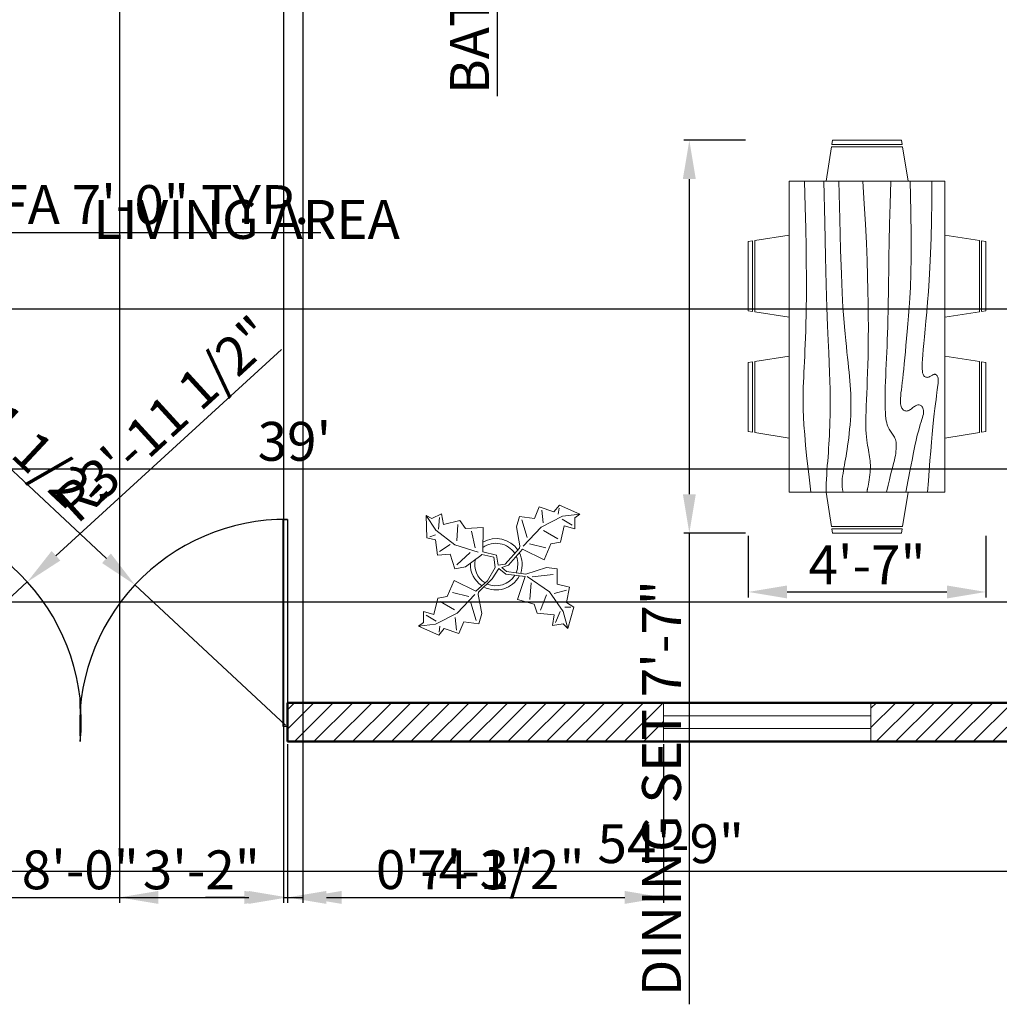
# Model space of a CAD drawing. Units: inches. Extents: x 61993 to 62774, y 55335 to 55871.
# Tile 2 of 6: x 62247 to 62474, y 55335 to 55563. Entities that reach past the tile are written whole.
import ezdxf

# ---------------------------------------------------------------- set-up
doc = ezdxf.new("R2010")
doc.units = ezdxf.units.IN
for name, color, linetype, lineweight in [('A-ANNO-DIMS', 2, 'Continuous', 18), ('A-AREA-IDEN', 7, 'Continuous', 25), ('A-DOOR', 3, 'Continuous', 25), ('A-FURN', 9, 'Continuous', 18), ('A-FURN-PLNT', 94, 'Continuous', 13), ('A-GLAZ', 4, 'Continuous', 18), ('A-WALL', 7, 'Continuous', 50)]:
    doc.layers.add(name, color=color, linetype=linetype, lineweight=lineweight)
doc.layers.add('A-WALL-PATT', color=40, linetype='Continuous', lineweight=13, true_color=0xf8d731)
doc.styles.get("Standard").update_dxf_attribs({"font": 'arial.ttf'})
doc.dimstyles.new('ISO-25', dxfattribs={"dimtxt": 9, "dimasz": 9, "dimexe": 1.25, "dimexo": 0.625, "dimtad": 1, "dimdec": 1, "dimrnd": 9, "dimlunit": 3, "dimtxsty": 'Standard', "dimcen": 2.5, "dimadec": 0, "dimazin": 0, "dimtfac": 1, "dimtdec": 1, "dimtmove": 0, "dimatfit": 3, "dimfxl": 1, "dimarcsym": 0})

# ---------------------------------------------------------------- blocks, each defined once
blk = doc.blocks.new('*D12')
at = {"layer": 'A-ANNO-DIMS', "color": 0, "lineweight": -2, "transparency": 16777216}
for p, q in [((62077.82, 55405.58), (62077.82, 55460.37)), ((62086.82, 55459.12), (62534.69, 55459.12)), ((62543.69, 55405.58), (62543.69, 55460.37))]:
    blk.add_line(p, q, dxfattribs=at)
at = {"layer": 'A-ANNO-DIMS', "color": 0, "transparency": 16777216}
for points in [[(62086.82, 55460.62), (62086.82, 55457.62), (62077.82, 55459.12)], [(62534.69, 55460.62), (62534.69, 55457.62), (62543.69, 55459.12)]]:
    blk.add_solid(points, dxfattribs=at)
at = {"layer": 'Defpoints', "color": 0, "transparency": 16777216}
for p in [(62543.69, 55459.12), (62077.82, 55404.96), (62543.69, 55404.96)]:
    blk.add_point(p, dxfattribs=at)
at = {"layer": 'A-ANNO-DIMS', "color": 0, "transparency": 16777216, "insert": (62310.76, 55464.35), "char_height": 9, "attachment_point": 5}
blk.add_mtext("39'", dxfattribs=at)
blk = doc.blocks.new('Plant - Rubber or Philodendron')
for p, q in [((13.3837, 12.301), (14.68, 13.9039)), ((14.68, 13.9039), (19.3848, 11.8146)), ((-16.2005, 11.4774), (-13.9899, 8.1064)), ((-16.2005, 11.4774), (-14.8639, 10.7964)), ((-16.0159, 6.3329), (-16.2005, 11.4774)), ((-14.8639, 10.7964), (-12.6195, 11.8975)), ((-12.6195, 11.8975), (-12.1909, 9.4345)), ((8.8871, 10.7908), (9.9809, 13.4933)), ((9.9809, 13.4933), (13.3837, 12.301)), ((10.5828, 12.6946), (10.8893, 9.7953)), ((14.5816, 13.2037), (14.3848, 11.8033)), ((19.3848, 11.8146), (15.3859, 11.3055)), ((19.3848, 11.8146), (18.1868, 10.9119)), ((-13.3174, 8.325), (-13.0735, 11.0065)), ((-12.1909, 9.4345), (-8.3829, 10.3)), ((-8.8369, 9.409), (-9.0894, 5.6095)), ((-8.3829, 10.3), (-7.0549, 8.501)), ((4.6914, 8.8812), (5.3859, 11.2828)), ((5.3859, 11.2828), (8.8871, 10.7908)), ((5.9878, 10.4842), (7.1971, 6.3869)), ((15.3859, 11.3055), (10.3916, 8.7942)), ((15.2875, 10.6053), (17.5907, 9.2105)), ((18.1868, 10.9119), (18.1925, 8.4119)), ((-15.3434, 6.5514), (-13.9984, 6.9884)), ((-13.9899, 8.1064), (-9.5434, 4.7185)), ((-7.0549, 8.501), (-3.0284, 8.6941)), ((-4.8529, 4.012), (-5.7184, 7.82)), ((-3.0284, 8.6941), (-3.0709, 3.1041)), ((4.6914, 8.8812), (5.5014, 4.4831)), ((10.3916, 8.7942), (6.2847, 4.4028)), ((14.2977, 6.1031), (10.9934, 7.9956)), ((15.7909, 9.1065), (14.8995, 5.3044)), ((18.1925, 8.4119), (15.7909, 9.1065)), ((-14.0069, 5.8704), (-16.0159, 6.3329)), ((-13.5868, 2.2894), (-14.0069, 5.8704)), ((-13.1329, 3.1804), (-10.6614, 4.727)), ((-9.5434, 4.7185), (-4.1917, 2.9888)), ((7.7005, 4.8881), (11.5025, 3.9967)), ((12.7005, 4.8994), (11.1089, 1.1958)), ((14.8995, 5.3044), (12.7005, 4.8994)), ((-10.6784, 2.491), (-13.5868, 2.2894)), ((-9.5858, -0.8715), (-10.6784, 2.491)), ((-9.1318, 0.0195), (-5.9793, 2.9025)), ((-3.5248, 2.2131), (-3.3011, 2.4355)), ((-3.3011, 2.4355), (-0.5306, 1.7947)), ((-3.0709, 3.1041), (0.0797, 2.3163)), ((0.0797, 2.3163), (0.4866, -0.031)), ((2.1141, 0.2298), (5.4346, 3.9146)), ((6.1032, 3.6844), (2.8262, -0.031)), ((5.4346, 3.9146), (5.5014, 4.4831)), ((11.1089, 1.1958), (6.1032, 3.6844)), ((-7.1228, -0.443), (-3.5248, 2.2131)), ((-0.5306, 1.7947), (-0.2255, -0.5527)), ((-0.5306, 1.7947), (-0.5306, 1.7947)), ((0.4866, -0.031), (2.1141, 0.2298)), ((-7.1228, -0.443), (-9.5858, -0.8715)), ((-2.019, -3.6148), (-0.2255, -0.5527)), ((-0.9375, -3.1608), (0.5883, -0.8135)), ((0.5883, -0.8135), (2.2447, -2.0916)), ((2.8262, -0.031), (1.3003, -0.5527)), ((1.3003, -0.5527), (2.4193, -1.4655)), ((2.2447, -2.0916), (6.7108, -2.6626)), ((2.4193, -1.4655), (6.895, -2.1175)), ((11.6605, -0.5413), (6.895, -2.1175)), ((8.3544, -2.7453), (13.1973, -2.1704)), ((11.6605, -0.5413), (14.1354, -0.8948)), ((14.1354, -0.8948), (14.1354, -4.4304)), ((-11.3237, -7.2629), (-9.7321, -3.5593)), ((-9.7321, -3.5593), (-4.7264, -6.0479)), ((-2.019, -3.6148), (-4.7264, -6.0479)), ((-4.0579, -6.2781), (-0.9375, -3.1608)), ((4.943, -7.9659), (6.7108, -2.6626)), ((12.3677, -6.1981), (7.219, -2.6772)), ((8.125, -4.0768), (7.7715, -7.9659)), ((14.1354, -4.4304), (16.9638, -5.1375)), ((-6.3237, -7.2516), (-10.1257, -6.3602)), ((-9.0148, -11.1577), (-4.9047, -6.8122)), ((-4.1246, -6.8466), (-4.0579, -6.2781)), ((15.5496, -10.7943), (12.3677, -6.1981)), ((16.2567, -5.8446), (13.4283, -6.5517)), ((16.9638, -5.1375), (16.2567, -8.673)), ((-14.4141, -11.4699), (-13.5228, -7.6679)), ((-13.5228, -7.6679), (-11.3237, -7.2629)), ((-12.921, -8.4665), (-9.6166, -10.359)), ((-4.611, -12.8477), (-5.8203, -8.7504)), ((-3.3146, -11.2447), (-4.1246, -6.8466)), ((8.8321, -9.0266), (4.943, -7.9659)), ((9.5392, -11.1479), (8.8321, -9.0266)), ((10.2463, -10.4408), (11.6605, -6.9053)), ((16.2567, -8.673), (18.0245, -9.7337)), ((-16.8157, -10.7754), (-14.4141, -11.4699)), ((-16.8101, -13.2754), (-16.8157, -10.7754)), ((-14.0091, -13.669), (-9.0148, -11.1577)), ((-3.3146, -11.2447), (-4.0092, -13.6463)), ((13.4283, -11.5015), (9.5392, -11.1479)), ((14.8425, -10.7943), (13.7819, -13.2692)), ((16.6103, -14.6834), (15.5496, -10.7943)), ((17.3174, -9.7337), (15.9032, -9.7337)), ((18.0245, -9.7337), (16.6103, -14.6834)), ((-18.008, -14.1781), (-16.8101, -13.2754)), ((-18.008, -14.1781), (-14.0091, -13.669)), ((-13.9107, -12.9688), (-16.2139, -11.574)), ((-9.206, -15.0581), (-9.5126, -12.1588)), ((-7.5103, -13.1543), (-8.6042, -15.8568)), ((-4.0092, -13.6463), (-7.5103, -13.1543)), ((13.0748, -13.9763), (13.4283, -11.5015)), ((15.5496, -13.6228), (13.0748, -13.9763)), ((16.6103, -14.6834), (15.5496, -13.6228)), ((-13.3032, -16.2674), (-18.008, -14.1781)), ((-12.0069, -14.6645), (-13.3032, -16.2674)), ((-13.2048, -15.5672), (-13.008, -14.1668)), ((-8.6042, -15.8568), (-12.0069, -14.6645))]:
    blk.add_line(p, q)
for centre, radius, start, end in [((0, 0), 6.1275, 34.37569, 120.1028), ((-0.0601, -0.2075), 5.2461, 33.82192, 124.9414), ((-0.098, 0.1364), 6.1288, 341.2017, 26.09184), ((0.0308, 0.1664), 6, 178.6147, 235.1169), ((0.0308, 0.1664), 5, 168.1647, 238.6725), ((-0.2664, 0.1682), 5.2775, 338.4094, 20.03007), ((-0.0234, 0.3825), 6.1492, 242.5812, 331.2714), ((-0.1102, 0.4886), 5.2883, 247.3711, 327.472)]:
    blk.add_arc(centre, radius, start, end)
blk = doc.blocks.new('Dining Set - 36 x 72 in.')
for p, q in [((-22, 27.5), (-22.1562, 26.50042)), ((-22, 27.5), (-6, 27.5)), ((-5.8437, 26.49966), (-6, 27.5)), ((6, 27.5), (5.8438, 26.50042)), ((6, 27.5), (22, 27.5)), ((22.1563, 26.49966), (22, 27.5)), ((-22.2343, 26.00059), (-23.4847, 17.99762)), ((-22.2304, 26), (-5.7608, 26)), ((-5.8416, 26.5), (-22.1534, 26.5)), ((-4.5152, 17.99762), (-5.7655, 25.99926)), ((5.7657, 26.00059), (4.5153, 17.99762)), ((5.7696, 26), (22.2392, 26)), ((22.1584, 26.5), (5.8466, 26.5)), ((23.4848, 17.99762), (22.2345, 25.99926)), ((36, 18), (-36, 18)), ((-36, 18), (-36, -18)), ((36, -18), (36, 18)), ((-44.0006, 8.23428), (-35.9976, 9.48474)), ((44.0006, 8.23428), (35.9976, 9.48474)), ((-45.5, 8), (-44.5004, 8.15617)), ((-45.5, 8), (-45.5, -8)), ((-44.5, -8.15843), (-44.5, 8.15338)), ((-44, 8.23041), (-44, -8.23915)), ((44, 8.23041), (44, -8.23915)), ((44.5, -8.15843), (44.5, 8.15338)), ((45.5, 8), (44.5005, 8.15617)), ((45.5, 8), (45.5, -8)), ((-44.4997, -8.15631), (-45.5, -8)), ((-35.9976, -9.48476), (-43.9993, -8.2345)), ((35.9976, -9.48476), (43.9993, -8.2345)), ((44.4997, -8.15631), (45.5, -8)), ((-36, -18), (36, -18)), ((-22.2343, -26.0006), (-23.4847, -17.99762)), ((-4.5152, -17.99762), (-5.7655, -25.99928)), ((5.7657, -26.0006), (4.5153, -17.99762)), ((23.4848, -17.99762), (22.2345, -25.99928)), ((-22.2304, -26), (-5.7608, -26)), ((-22, -27.5), (-22.1562, -26.50044)), ((-5.8416, -26.5), (-22.1534, -26.5)), ((-5.8437, -26.49967), (-6, -27.5)), ((5.7696, -26), (22.2392, -26)), ((6, -27.5), (5.8438, -26.50044)), ((22.1584, -26.5), (5.8466, -26.5)), ((22.1563, -26.49967), (22, -27.5)), ((-22, -27.5), (-6, -27.5)), ((6, -27.5), (22, -27.5))]:
    blk.add_line(p, q)
for points in [[(-36, 15), (-31.1772, 14.97754), (-26.8079, 14.91406), (-22.8538, 14.81543), (-19.276, 14.6875), (-16.0362, 14.53613), (-13.0957, 14.36718), (-10.4159, 14.18652), (-7.9583, 14), (-5.6904, 13.81315), (-3.6035, 13.63021), (-1.6954, 13.45508), (0.0365, 13.29166), (1.5945, 13.14388), (2.9811, 13.01562), (4.1988, 12.9108), (5.25, 12.83333), (6.1393, 12.78613), (6.8802, 12.76823), (7.4883, 12.77767), (7.9792, 12.8125), (8.3685, 12.87077), (8.6719, 12.95052), (8.9049, 13.0498), (9.0833, 13.16666), (9.2205, 13.29899), (9.3216, 13.44401), (9.3895, 13.59879), (9.4271, 13.76041), (9.4373, 13.92594), (9.4232, 14.09245), (9.3875, 14.257), (9.3333, 14.41666), (9.2638, 14.56917), (9.1836, 14.71484), (9.0975, 14.85465), (9.0104, 14.98958), (8.9272, 15.1206), (8.8529, 15.2487), (8.7922, 15.37483), (8.75, 15.5), (8.7305, 15.62467), (8.7344, 15.74739), (8.7617, 15.86621), (8.8125, 15.97916), (8.8867, 16.08431), (8.9844, 16.17968), (9.1055, 16.26334), (9.25, 16.33333), (9.4189, 16.38802), (9.6172, 16.42708), (9.8506, 16.45052), (10.125, 16.45833), (10.4463, 16.45052), (10.8203, 16.42708), (11.2529, 16.38802), (11.75, 16.33333), (12.3184, 16.26318), (12.9694, 16.17838), (13.7151, 16.07991), (14.5677, 15.96875), (15.5395, 15.84586), (16.6426, 15.71224), (17.8893, 15.56884), (19.2917, 15.41666), (20.859, 15.25667), (22.5879, 15.08984), (24.4721, 14.91715), (26.5052, 14.73958), (28.6809, 14.5581), (30.9929, 14.3737), (33.4347, 14.18733), (36, 14)], [(-36, 10), (-28.9766, 10.14274), (-23.1725, 10.20442), (-18.4241, 10.19775), (-14.5677, 10.13541), (-11.4399, 10.03011), (-8.877, 9.89453), (-6.7154, 9.74137), (-4.7917, 9.58333), (-2.9698, 9.43082), (-1.2246, 9.28515), (0.4415, 9.14534), (2.026, 9.01041), (3.5266, 8.87939), (4.9408, 8.7513), (6.266, 8.62516), (7.5, 8.5), (8.6411, 8.37549), (9.6914, 8.2539), (10.6538, 8.13818), (11.5312, 8.03125), (12.3267, 7.93603), (13.043, 7.85547), (13.6831, 7.79248), (14.25, 7.75), (14.7471, 7.7303), (15.1797, 7.73307), (15.5537, 7.75732), (15.875, 7.80208), (16.1494, 7.86637), (16.3828, 7.94922), (16.5811, 8.04964), (16.75, 8.16666), (16.8944, 8.29915), (17.0143, 8.44531), (17.1089, 8.60319), (17.1771, 8.77083), (17.218, 8.94629), (17.2305, 9.1276), (17.2137, 9.31282), (17.1667, 9.5), (17.0895, 9.6875), (16.987, 9.875), (16.8649, 10.0625), (16.7292, 10.25), (16.5856, 10.4375), (16.4401, 10.625), (16.2985, 10.8125), (16.1667, 11), (16.05, 11.18733), (15.9518, 11.3737), (15.8752, 11.5581), (15.8229, 11.73958), (15.798, 11.91715), (15.8034, 12.08984), (15.842, 12.25667), (15.9167, 12.41666), (16.0295, 12.56836), (16.1784, 12.70833), (16.3605, 12.83268), (16.5729, 12.9375), (16.8127, 13.01888), (17.0768, 13.07291), (17.3625, 13.0957), (17.6667, 13.08333), (17.9894, 13.03312), (18.3418, 12.94726), (18.7382, 12.82918), (19.1927, 12.68229), (19.7195, 12.51001), (20.3327, 12.31575), (21.0465, 12.10294), (21.875, 11.875), (22.8357, 11.63354), (23.959, 11.37304), (25.2786, 11.08618), (26.8282, 10.76562), (28.6414, 10.40405), (30.752, 9.99414), (33.1936, 9.52856), (36, 9)], [(-36, 5.5), (-30.7157, 5.3348), (-26.069, 5.20963), (-21.9946, 5.11767), (-18.4271, 5.05208), (-15.3009, 5.00602), (-12.5508, 4.97265), (-10.1112, 4.94515), (-7.9167, 4.91666), (-5.909, 4.88167), (-4.0586, 4.83984), (-2.3429, 4.79215), (-0.7396, 4.73958), (0.7739, 4.6831), (2.22, 4.6237), (3.6213, 4.56233), (5, 4.5), (6.373, 4.43782), (7.7344, 4.3776), (9.0723, 4.32129), (10.375, 4.27083), (11.6309, 4.22819), (12.8281, 4.19531), (13.9551, 4.17415), (15, 4.16666), (15.954, 4.17448), (16.819, 4.19791), (17.6001, 4.23698), (18.3021, 4.29166), (18.9299, 4.36198), (19.4883, 4.44791), (19.9823, 4.54948), (20.4167, 4.66666), (20.7969, 4.79899), (21.1302, 4.94401), (21.4245, 5.09879), (21.6875, 5.26041), (21.9271, 5.42594), (22.1511, 5.59245), (22.3672, 5.757), (22.5834, 5.91666), (22.8065, 6.06868), (23.0404, 6.21093), (23.2879, 6.34147), (23.5521, 6.45833), (23.8358, 6.55957), (24.142, 6.64323), (24.4735, 6.70735), (24.8334, 6.75), (25.2235, 6.76969), (25.642, 6.76692), (26.0858, 6.74267), (26.5521, 6.69791), (27.0379, 6.63362), (27.5404, 6.55078), (28.0565, 6.45036), (28.5834, 6.33333), (29.1242, 6.19987), (29.7071, 6.04687), (30.3661, 5.87044), (31.1354, 5.66666), (32.0493, 5.43164), (33.142, 5.16146), (34.4475, 4.85221), (36, 4.5)], [(-36, -1), (-30.7915, -0.6591), (-26.0195, -0.38216), (-21.6519, -0.16284), (-17.6563, 0.00521), (-14.0005, 0.12833), (-10.6523, 0.21289), (-7.5796, 0.26522), (-4.75, 0.29166), (-2.134, 0.29793), (0.2878, 0.28711), (2.5317, 0.26163), (4.6146, 0.22396), (6.5529, 0.17651), (8.3633, 0.12174), (10.0623, 0.06209), (11.6667, 0), (13.1899, -0.06201), (14.6341, -0.1211), (15.9982, -0.17432), (17.2813, -0.21875), (18.4823, -0.25147), (19.6003, -0.26953), (20.6343, -0.27002), (21.5834, -0.25), (22.4481, -0.20768), (23.2357, -0.14584), (23.9549, -0.06836), (24.6146, 0.02083), (25.2235, 0.11784), (25.7904, 0.21875), (26.3241, 0.31966), (26.8334, 0.41666), (27.3265, 0.50618), (27.8099, 0.58593), (28.2894, 0.65397), (28.7709, 0.70833), (29.2601, 0.74707), (29.763, 0.76823), (30.2855, 0.76985), (30.8334, 0.75), (31.4088, 0.70784), (31.9994, 0.64713), (32.589, 0.57275), (33.1615, 0.48958), (33.7008, 0.4025), (34.1908, 0.3164), (34.6153, 0.23616), (34.9584, 0.16666), (35.2099, 0.11165), (35.3848, 0.07031), (35.504, 0.04069), (35.5886, 0.02083), (35.6594, 0.00879), (35.7377, 0.0026), (35.8442, 0.00032), (36, 0)], [(-36, -6.5), (-27.1843, -6.31267), (-20.084, -6.1263), (-14.469, -5.9419), (-10.1094, -5.76042), (-6.7752, -5.58285), (-4.2363, -5.41016), (-2.2629, -5.24333), (-0.625, -5.08334), (0.8708, -4.93099), (2.2715, -4.78646), (3.5872, -4.64974), (4.8281, -4.52084), (6.0046, -4.39974), (7.127, -4.28646), (8.2053, -4.18099), (9.25, -4.08334), (10.2705, -3.99382), (11.2734, -3.91407), (12.2647, -3.84603), (13.25, -3.79167), (14.2354, -3.75293), (15.2266, -3.73177), (16.2295, -3.73015), (17.25, -3.75), (18.2912, -3.79248), (19.3451, -3.85547), (20.4009, -3.93604), (21.4479, -4.03125), (22.4754, -4.13819), (23.4727, -4.25391), (24.4289, -4.37549), (25.3334, -4.5), (26.1785, -4.62492), (26.9694, -4.74935), (27.7145, -4.87281), (28.4219, -4.99479), (29.1, -5.11483), (29.7572, -5.23242), (30.4016, -5.34709), (31.0417, -5.45834), (31.6837, -5.56437), (32.3262, -5.65821), (32.9658, -5.73153), (33.599, -5.77604), (34.2224, -5.78345), (34.8327, -5.74545), (35.4264, -5.65373), (36, -5.5)], [(-36, -10), (-26.4022, -9.81299), (-18.4675, -9.62891), (-11.9839, -9.45069), (-6.7396, -9.28125), (-2.5226, -9.12354), (0.8789, -8.98047), (3.6769, -8.85498), (6.0833, -8.75), (8.2767, -8.66765), (10.3021, -8.60677), (12.1712, -8.56543), (13.8958, -8.54167), (15.4876, -8.53353), (16.9583, -8.53907), (18.3197, -8.55632), (19.5834, -8.58334), (20.7616, -8.61841), (21.8685, -8.66081), (22.9188, -8.71004), (23.9271, -8.76563), (24.9081, -8.82707), (25.8763, -8.89388), (26.8465, -8.96558), (27.8334, -9.04167), (28.8474, -9.12118), (29.8828, -9.20117), (30.93, -9.27824), (31.9792, -9.34896), (33.0205, -9.40991), (34.0443, -9.45768), (35.0407, -9.48885), (36, -9.5)], [(-36, -14.5), (-30.0881, -14.33513), (-25.0332, -14.21224), (-20.7312, -14.12647), (-17.0781, -14.07292), (-13.97, -14.04671), (-11.3027, -14.04297), (-8.9724, -14.05681), (-6.875, -14.08334), (-4.9224, -14.11833), (-3.0905, -14.16016), (-1.3709, -14.20785), (0.2448, -14.26042), (1.7647, -14.3169), (3.1973, -14.3763), (4.5507, -14.43767), (5.8333, -14.5), (7.0554, -14.5621), (8.235, -14.62175), (9.3922, -14.67652), (10.5469, -14.72396), (11.7192, -14.76164), (12.929, -14.78711), (14.1965, -14.79794), (15.5417, -14.79167), (16.9933, -14.76424), (18.6152, -14.70508), (20.4804, -14.60197), (22.6615, -14.44271), (25.2312, -14.21509), (28.2624, -13.9069), (31.8277, -13.50594), (36, -13)]]:
    blk.add_lwpolyline(points)
blk = doc.blocks.new('*D28')
at = {"layer": 'A-ANNO-DIMS', "color": 0, "lineweight": -2, "transparency": 16777216}
for p, q in [((62067.57, 55395.33), (62067.57, 55364.68)), ((62728.19, 55395.33), (62728.19, 55364.68)), ((62076.57, 55365.93), (62719.19, 55365.93))]:
    blk.add_line(p, q, dxfattribs=at)
at = {"layer": 'A-ANNO-DIMS', "color": 0, "transparency": 16777216}
for points in [[(62076.57, 55367.43), (62076.57, 55364.43), (62067.57, 55365.93)], [(62719.19, 55367.43), (62719.19, 55364.43), (62728.19, 55365.93)]]:
    blk.add_solid(points, dxfattribs=at)
at = {"layer": 'Defpoints', "color": 0, "transparency": 16777216}
for p in [(62067.57, 55395.96), (62728.19, 55395.96), (62728.19, 55365.93)]:
    blk.add_point(p, dxfattribs=at)
at = {"layer": 'A-ANNO-DIMS', "color": 0, "transparency": 16777216, "insert": (62397.88, 55371.15), "char_height": 9, "attachment_point": 5}
blk.add_mtext('54\'-9"', dxfattribs=at)
blk = doc.blocks.new('WIN-48IN')
for p, q in [((0, 9), (0, 0)), ((48, 9), (48, 0)), ((48, 6), (0, 6)), ((48, 3), (0, 3))]:
    blk.add_line(p, q)
blk = doc.blocks.new('*D42')
at = {"layer": 'A-ANNO-DIMS', "color": 0, "lineweight": -2, "transparency": 16777216}
for p, q in [((62130.08, 55525.89), (62130.08, 55512.67)), ((62214.08, 55525.89), (62214.08, 55512.67)), ((62139.08, 55513.92), (62205.08, 55513.92)), ((62214.08, 55513.92), (62316.87, 55513.92))]:
    blk.add_line(p, q, dxfattribs=at)
at = {"layer": 'A-ANNO-DIMS', "color": 0, "transparency": 16777216}
for points in [[(62139.08, 55515.42), (62139.08, 55512.42), (62130.08, 55513.92)], [(62205.08, 55515.42), (62205.08, 55512.42), (62214.08, 55513.92)]]:
    blk.add_solid(points, dxfattribs=at)
at = {"layer": 'Defpoints', "color": 0, "transparency": 16777216}
for p in [(62130.08, 55526.52), (62214.08, 55526.52), (62214.08, 55513.92)]:
    blk.add_point(p, dxfattribs=at)
at = {"layer": 'A-ANNO-DIMS', "color": 0, "transparency": 16777216, "insert": (62269.98, 55519.2), "char_height": 9, "attachment_point": 5}
blk.add_mtext('SOFA 7\'-0" TYP.', dxfattribs=at)
blk = doc.blocks.new('*D48')
at = {"layer": 'A-ANNO-DIMS', "color": 0, "lineweight": -2, "transparency": 16777216}
for p, q in [((62349.32, 55701.42), (62358.94, 55701.42)), ((62357.69, 55692.42), (62357.69, 55650.42)), ((62349.32, 55641.42), (62358.94, 55641.42)), ((62357.69, 55641.42), (62357.69, 55545.48))]:
    blk.add_line(p, q, dxfattribs=at)
at = {"layer": 'A-ANNO-DIMS', "color": 0, "transparency": 16777216}
for points in [[(62356.19, 55692.42), (62359.19, 55692.42), (62357.69, 55701.42)], [(62356.19, 55650.42), (62359.19, 55650.42), (62357.69, 55641.42)]]:
    blk.add_solid(points, dxfattribs=at)
at = {"layer": 'Defpoints', "color": 0, "transparency": 16777216}
for p in [(62348.69, 55701.42), (62348.69, 55641.42), (62357.69, 55641.42)]:
    blk.add_point(p, dxfattribs=at)
at = {"layer": 'A-ANNO-DIMS', "color": 0, "transparency": 16777216, "insert": (62352.47, 55588.95), "char_height": 9, "attachment_point": 5, "rotation": 90}
blk.add_mtext('BATHTUB 5\'-0"', dxfattribs=at)
blk = doc.blocks.new('*D54')
at = {"layer": 'A-ANNO-DIMS', "color": 0, "lineweight": -2, "transparency": 16777216}
for p, q in [((62415.2, 55535.27), (62400.93, 55535.27)), ((62402.18, 55526.27), (62402.18, 55453.27)), ((62415.2, 55444.27), (62400.93, 55444.27)), ((62402.18, 55444.27), (62402.18, 55335.1))]:
    blk.add_line(p, q, dxfattribs=at)
at = {"layer": 'A-ANNO-DIMS', "color": 0, "transparency": 16777216}
for points in [[(62400.68, 55526.27), (62403.68, 55526.27), (62402.18, 55535.27)], [(62400.68, 55453.27), (62403.68, 55453.27), (62402.18, 55444.27)]]:
    blk.add_solid(points, dxfattribs=at)
at = {"layer": 'Defpoints', "color": 0, "transparency": 16777216}
for p in [(62415.83, 55535.27), (62402.18, 55444.27), (62415.83, 55444.27)]:
    blk.add_point(p, dxfattribs=at)
at = {"layer": 'A-ANNO-DIMS', "color": 0, "transparency": 16777216, "insert": (62396.9, 55385.18), "char_height": 9, "attachment_point": 5, "rotation": 90}
blk.add_mtext('DINING SET 7\'-7"', dxfattribs=at)
blk = doc.blocks.new('*D55')
at = {"layer": 'A-ANNO-DIMS', "color": 0, "lineweight": -2, "transparency": 16777216}
for p, q in [((62415.83, 55443.64), (62415.83, 55429.37)), ((62470.83, 55443.64), (62470.83, 55429.37)), ((62424.83, 55430.62), (62461.83, 55430.62))]:
    blk.add_line(p, q, dxfattribs=at)
at = {"layer": 'A-ANNO-DIMS', "color": 0, "transparency": 16777216}
for points in [[(62424.83, 55432.12), (62424.83, 55429.12), (62415.83, 55430.62)], [(62461.83, 55432.12), (62461.83, 55429.12), (62470.83, 55430.62)]]:
    blk.add_solid(points, dxfattribs=at)
at = {"layer": 'Defpoints', "color": 0, "transparency": 16777216}
for p in [(62415.83, 55444.27), (62470.83, 55444.27), (62470.83, 55430.62)]:
    blk.add_point(p, dxfattribs=at)
at = {"layer": 'A-ANNO-DIMS', "color": 0, "transparency": 16777216, "insert": (62443.33, 55435.74), "char_height": 9, "attachment_point": 5}
blk.add_mtext('4\'-7"', dxfattribs=at)
blk = doc.blocks.new('*D60')
at = {"layer": 'A-ANNO-DIMS', "color": 0, "lineweight": -2, "transparency": 16777216}
for p, q in [((62213.17, 55395.33), (62213.17, 55358.61)), ((62309.17, 55395.33), (62309.17, 55358.61)), ((62222.17, 55359.86), (62300.17, 55359.86))]:
    blk.add_line(p, q, dxfattribs=at)
at = {"layer": 'A-ANNO-DIMS', "color": 0, "transparency": 16777216}
for points in [[(62222.17, 55361.36), (62222.17, 55358.36), (62213.17, 55359.86)], [(62300.17, 55361.36), (62300.17, 55358.36), (62309.17, 55359.86)]]:
    blk.add_solid(points, dxfattribs=at)
at = {"layer": 'Defpoints', "color": 0, "transparency": 16777216}
for p in [(62213.17, 55395.96), (62309.17, 55395.96), (62309.17, 55359.86)]:
    blk.add_point(p, dxfattribs=at)
at = {"layer": 'A-ANNO-DIMS', "color": 0, "transparency": 16777216, "insert": (62261.17, 55365.08), "char_height": 9, "attachment_point": 5}
blk.add_mtext('8\'-0"', dxfattribs=at)
blk = doc.blocks.new('*D62')
at = {"layer": 'A-ANNO-DIMS', "color": 0, "lineweight": -2, "transparency": 16777216}
for p, q in [((62309.17, 55395.33), (62309.17, 55358.61)), ((62396.22, 55395.33), (62396.22, 55358.61)), ((62318.17, 55359.86), (62387.22, 55359.86))]:
    blk.add_line(p, q, dxfattribs=at)
at = {"layer": 'A-ANNO-DIMS', "color": 0, "transparency": 16777216}
for points in [[(62318.17, 55361.36), (62318.17, 55358.36), (62309.17, 55359.86)], [(62387.22, 55361.36), (62387.22, 55358.36), (62396.22, 55359.86)]]:
    blk.add_solid(points, dxfattribs=at)
at = {"layer": 'Defpoints', "color": 0, "transparency": 16777216}
for p in [(62309.17, 55395.96), (62396.22, 55395.96), (62396.22, 55359.86)]:
    blk.add_point(p, dxfattribs=at)
at = {"layer": 'A-ANNO-DIMS', "color": 0, "transparency": 16777216, "insert": (62352.69, 55365.08), "char_height": 9, "attachment_point": 5}
blk.add_mtext('7\'-3"', dxfattribs=at)
blk = doc.blocks.new('*D71')
at = {"layer": 'A-ANNO-DIMS', "color": 0, "lineweight": -2, "transparency": 16777216}
for p, q in [((62308.19, 55575.33), (62308.19, 55358.61)), ((62270.23, 55570.83), (62270.23, 55358.61)), ((62279.23, 55359.86), (62299.19, 55359.86))]:
    blk.add_line(p, q, dxfattribs=at)
at = {"layer": 'A-ANNO-DIMS', "color": 0, "transparency": 16777216}
for points in [[(62279.23, 55361.36), (62279.23, 55358.36), (62270.23, 55359.86)], [(62299.19, 55361.36), (62299.19, 55358.36), (62308.19, 55359.86)]]:
    blk.add_solid(points, dxfattribs=at)
at = {"layer": 'Defpoints', "color": 0, "transparency": 16777216}
for p in [(62308.19, 55575.96), (62270.23, 55571.46), (62308.19, 55359.86)]:
    blk.add_point(p, dxfattribs=at)
at = {"layer": 'A-ANNO-DIMS', "color": 0, "transparency": 16777216, "insert": (62289.21, 55365.08), "char_height": 9, "attachment_point": 5}
blk.add_mtext('3\'-2"', dxfattribs=at)
blk = doc.blocks.new('*D74')
at = {"layer": 'A-ANNO-DIMS', "color": 0, "lineweight": -2, "transparency": 16777216}
for p, q in [((62032.09, 55580.46), (62032.09, 55589.46)), ((62547.57, 55571.46), (62030.84, 55571.46)), ((62032.09, 55571.46), (62032.09, 55568.46)), ((62547.57, 55568.46), (62030.84, 55568.46)), ((62032.09, 55559.46), (62032.09, 55525.28))]:
    blk.add_line(p, q, dxfattribs=at)
at = {"layer": 'A-ANNO-DIMS', "color": 0, "transparency": 16777216}
for points in [[(62030.59, 55580.46), (62033.59, 55580.46), (62032.09, 55571.46)], [(62030.59, 55559.46), (62033.59, 55559.46), (62032.09, 55568.46)]]:
    blk.add_solid(points, dxfattribs=at)
at = {"layer": 'Defpoints', "color": 0, "transparency": 16777216}
for p in [(62548.19, 55571.46), (62032.09, 55568.46), (62548.19, 55568.46)]:
    blk.add_point(p, dxfattribs=at)
at = {"layer": 'A-ANNO-DIMS', "color": 0, "transparency": 16777216, "insert": (62026.87, 55537.87), "char_height": 9, "attachment_point": 5, "rotation": 90}
blk.add_mtext('0\'-3"', dxfattribs=at)
blk = doc.blocks.new('*D75')
at = {"layer": 'A-ANNO-DIMS', "color": 0, "lineweight": -2, "transparency": 16777216}
for p, q in [((62308.19, 55806.33), (62308.19, 55358.61)), ((62312.69, 55806.33), (62312.69, 55358.61)), ((62299.19, 55359.86), (62290.19, 55359.86)), ((62308.19, 55359.86), (62312.69, 55359.86)), ((62321.69, 55359.86), (62376.84, 55359.86))]:
    blk.add_line(p, q, dxfattribs=at)
at = {"layer": 'A-ANNO-DIMS', "color": 0, "transparency": 16777216}
for points in [[(62299.19, 55361.36), (62299.19, 55358.36), (62308.19, 55359.86)], [(62321.69, 55361.36), (62321.69, 55358.36), (62312.69, 55359.86)]]:
    blk.add_solid(points, dxfattribs=at)
at = {"layer": 'Defpoints', "color": 0, "transparency": 16777216}
for p in [(62308.19, 55806.96), (62312.69, 55806.96), (62312.69, 55359.86)]:
    blk.add_point(p, dxfattribs=at)
at = {"layer": 'A-ANNO-DIMS', "color": 0, "transparency": 16777216, "insert": (62353.77, 55365.13), "char_height": 9, "attachment_point": 5}
blk.add_mtext('0\'-4 1/2"', dxfattribs=at)
blk = doc.blocks.new('*D80')
at = {"layer": 'A-ANNO-DIMS', "color": 0, "lineweight": -2, "transparency": 16777216}
for p, q in [((62558.29, 55496.17), (62030.84, 55496.17)), ((62032.09, 55437.26), (62032.09, 55487.17)), ((62558.29, 55428.26), (62030.84, 55428.26))]:
    blk.add_line(p, q, dxfattribs=at)
at = {"layer": 'A-ANNO-DIMS', "color": 0, "transparency": 16777216}
for points in [[(62030.59, 55487.17), (62033.59, 55487.17), (62032.09, 55496.17)], [(62030.59, 55437.26), (62033.59, 55437.26), (62032.09, 55428.26)]]:
    blk.add_solid(points, dxfattribs=at)
at = {"layer": 'Defpoints', "color": 0, "transparency": 16777216}
for p in [(62032.09, 55496.17), (62558.91, 55496.17), (62558.91, 55428.26)]:
    blk.add_point(p, dxfattribs=at)
at = {"layer": 'A-ANNO-DIMS', "color": 0, "transparency": 16777216, "insert": (62026.87, 55462.22), "char_height": 9, "attachment_point": 5, "rotation": 90}
blk.add_mtext('5\'-8"', dxfattribs=at)
blk = doc.blocks.new('*D85')
at = {"layer": 'A-ANNO-DIMS', "color": 0, "lineweight": -2, "transparency": 16777216}
for p, q in [((62307.76, 55486.75), (62255.54, 55439.01)), ((62213.67, 55400.72), (62248.9, 55432.93))]:
    blk.add_line(p, q, dxfattribs=at)
at = {"layer": 'A-ANNO-DIMS', "color": 0, "transparency": 16777216}
blk.add_solid([(62254.53, 55440.11), (62256.56, 55437.9), (62248.9, 55432.93)], dxfattribs=at)
at = {"layer": 'Defpoints', "color": 0, "transparency": 16777216}
for p in [(62248.9, 55432.93), (62213.67, 55400.72)]:
    blk.add_point(p, dxfattribs=at)
at = {"layer": 'A-ANNO-DIMS', "color": 0, "transparency": 16777216, "insert": (62281.41, 55469.81), "char_height": 9, "attachment_point": 5, "rotation": 42.4359}
blk.add_mtext('R3\'-11 1/2"', dxfattribs=at)
blk = doc.blocks.new('*D86')
at = {"layer": 'A-ANNO-DIMS', "color": 0, "lineweight": -2, "transparency": 16777216}
for p, q in [((62215.49, 55486.67), (62267.24, 55438.41)), ((62308.67, 55399.78), (62273.82, 55432.28))]:
    blk.add_line(p, q, dxfattribs=at)
at = {"layer": 'A-ANNO-DIMS', "color": 0, "transparency": 16777216}
blk.add_solid([(62268.26, 55439.51), (62266.21, 55437.32), (62273.82, 55432.28)], dxfattribs=at)
at = {"layer": 'Defpoints', "color": 0, "transparency": 16777216}
for p in [(62273.82, 55432.28), (62308.67, 55399.78)]:
    blk.add_point(p, dxfattribs=at)
at = {"layer": 'A-ANNO-DIMS', "color": 0, "transparency": 16777216, "insert": (62241.68, 55469.47), "char_height": 9, "attachment_point": 5, "rotation": 316.998}
blk.add_mtext('R3\'-11 1/2"', dxfattribs=at)

msp = doc.modelspace()

# ---------------------------------------------------------------- hatches: boundary and pattern name
at = {"layer": 'A-WALL-PATT'}
h = msp.add_hatch(dxfattribs=at)
h.set_pattern_fill('ANSI31', color=256)
h.paths.add_polyline_path([(62077.19, 55665.16), (62068.19, 55665.16), (62068.19, 55518.96), (62077.19, 55518.96), (62077.19, 55571.46), (62234.23, 55571.46), (62234.23, 55573.71, -0.007042), (62234.23, 55574.71), (62234.23, 55575.96), (62077.19, 55575.96)])
h.paths.add_polyline_path([(62077.19, 55806.96), (62138.51, 55806.96), (62138.51, 55815.96), (62068.19, 55815.96), (62068.19, 55713.16), (62077.19, 55713.16)])
h.paths.add_polyline_path([(62364.31, 55815.96), (62186.51, 55815.96), (62186.51, 55806.96), (62308.19, 55806.96), (62308.19, 55575.96), (62270.23, 55575.96), (62270.23, 55571.46), (62415.32, 55571.46), (62415.32, 55573.71, -0.007042), (62415.32, 55574.71), (62415.32, 55575.96), (62312.69, 55575.96), (62312.69, 55739.46), (62471.69, 55739.46), (62471.69, 55575.96), (62451.32, 55575.96), (62451.32, 55571.46), (62483.74, 55571.46), (62483.74, 55573.71, -0.007042), (62483.74, 55574.71), (62483.74, 55575.96), (62476.19, 55575.96), (62476.19, 55806.96), (62578.07, 55806.96), (62578.07, 55815.96), (62412.31, 55815.96), (62412.31, 55806.96), (62471.69, 55806.96), (62471.69, 55743.96), (62312.69, 55743.96), (62312.69, 55806.96), (62364.31, 55806.96)])
h.paths.add_polyline_path([(62728.19, 55815.96), (62626.07, 55815.96), (62626.07, 55806.96), (62719.19, 55806.96), (62719.19, 55739.46), (62728.19, 55739.46)])
h.paths.add_polyline_path([(62728.19, 55691.46), (62719.19, 55691.46), (62719.19, 55575.96), (62519.74, 55575.96), (62519.74, 55571.46), (62543.69, 55571.46), (62543.69, 55568.46), (62548.19, 55568.46), (62548.19, 55571.46), (62719.19, 55571.46), (62719.19, 55517.72), (62728.19, 55517.72)])
h.paths.add_polyline_path([(62599.31, 55404.96), (62548.19, 55404.96), (62548.19, 55532.46), (62546.94, 55532.46, -0.007042), (62545.94, 55532.46), (62543.69, 55532.46), (62543.69, 55404.96), (62444.22, 55404.96), (62444.22, 55395.96), (62599.31, 55395.96)])
h.paths.add_polyline_path([(62728.19, 55469.72), (62719.19, 55469.72), (62719.19, 55404.96), (62647.31, 55404.96), (62647.31, 55395.96), (62728.19, 55395.96)])
h.paths.add_polyline_path([(62396.22, 55404.96), (62309.17, 55404.96), (62309.17, 55395.96), (62396.22, 55395.96)])
h.paths.add_polyline_path([(62213.17, 55404.96), (62077.19, 55404.96), (62077.19, 55470.96), (62068.19, 55470.96), (62068.19, 55395.96), (62213.17, 55395.96)])

# ---------------------------------------------------------------- linework, layer by layer
at = {"layer": 'A-DOOR'}
for p, q in [((62308.17, 55399.43), (62308.17, 55447.43)), ((62308.17, 55447.43), (62309.17, 55447.43)), ((62309.17, 55447.43), (62309.17, 55404.96)), ((62261.17, 55403.59), (62261.17, 55405.49)), ((62309.17, 55399.43), (62308.17, 55399.43))]:
    msp.add_line(p, q, dxfattribs=at)
for centre, radius, start, end in [((62213.67, 55400.72), 47.74, 354.2723, 90.6001), ((62308.67, 55399.78), 47.65, 89.3988, 184.5963)]:
    msp.add_arc(centre, radius, start, end, dxfattribs=at)
at = {"layer": 'A-WALL'}
for p, q in [((62309.17, 55404.96), (62309.17, 55395.96)), ((62309.17, 55404.96), (62543.69, 55404.96)), ((62309.17, 55395.96), (62728.19, 55395.96))]:
    msp.add_line(p, q, dxfattribs=at)

# ---------------------------------------------------------------- block references
at = {"layer": 'A-FURN', "rotation": 270.0000000000041}
msp.add_blockref('Dining Set - 36 x 72 in.', (62443.33, 55489.77), dxfattribs=at)
at = {"layer": 'A-FURN-PLNT'}
msp.add_blockref('Plant - Rubber or Philodendron', (62357.45, 55436.85), dxfattribs=at)
at = {"layer": 'A-GLAZ'}
msp.add_blockref('WIN-48IN', (62396.22, 55395.96), dxfattribs=at)

# ---------------------------------------------------------------- texts
at = {"layer": 'A-AREA-IDEN', "insert": (62264.19, 55521.42), "char_height": 9, "attachment_point": 1}
msp.add_mtext_dynamic_manual_height_columns('LIVING AREA', width=116.6414, gutter_width=12.5, heights=[0], dxfattribs=at)

# ---------------------------------------------------------------- dimensions: what is measured, and where the dimension line sits
at = {"layer": 'A-ANNO-DIMS'}
for base, p1, p2, override, picture, middle in [((62312.69, 55359.86), (62308.19, 55806.96), (62312.69, 55806.96), {"dimdec": 1, "dimlfac": 1, "dimrnd": 0, "dimzin": 1, "dimdsep": 46, "dimlunit": 4, "dimfrac": 2}, '*D75', (62353.77, 55365.13)), ((62308.19, 55359.86), (62270.23, 55571.46), (62308.19, 55575.96), {"dimdec": 1, "dimlfac": 1, "dimrnd": 0, "dimzin": 1, "dimdsep": 46, "dimlunit": 4, "dimfrac": 2}, '*D71', (62289.21, 55365.08)), ((62543.69, 55459.12), (62077.82, 55404.96), (62543.69, 55404.96), {"dimclrd": 0, "dimclre": 0, "dimclrt": 0}, '*D12', (62310.76, 55464.35)), ((62470.83, 55430.62), (62415.83, 55444.27), (62470.83, 55444.27), {"dimdec": 1, "dimlfac": 1, "dimrnd": 0, "dimzin": 1, "dimdsep": 46, "dimlunit": 4, "dimfrac": 2}, '*D55', (62443.33, 55435.74)), ((62309.17, 55359.86), (62213.17, 55395.96), (62309.17, 55395.96), {"dimdec": 1, "dimlfac": 1, "dimrnd": 0, "dimzin": 1, "dimdsep": 46, "dimlunit": 4, "dimfrac": 2}, '*D60', (62261.17, 55365.08)), ((62396.2188, 55359.8565), (62309.1695, 55395.9565), (62396.2188, 55395.9565), {"dimdec": 1, "dimlfac": 1, "dimrnd": 0, "dimzin": 1, "dimdsep": 46, "dimlunit": 4, "dimfrac": 2}, '*D62', (62352.6941, 55365.0797))]:
    dim = msp.add_linear_dim(base=base, p1=p1, p2=p2, dimstyle='ISO-25', override=override, dxfattribs=at)
    dim.commit()
    dim.dimension.update_dxf_attribs({"geometry": picture, "text_midpoint": middle})
for base, p1, p2, text, picture, middle in [((62357.69, 55641.42), (62348.69, 55701.42), (62348.69, 55641.42), 'BATHTUB <>', '*D48', (62352.47, 55588.95)), ((62402.18, 55444.27), (62415.83, 55535.27), (62415.83, 55444.27), 'DINING SET <>', '*D54', (62396.9, 55385.18))]:
    dim = msp.add_linear_dim(base=base, p1=p1, p2=p2, angle=270, text=text, dimstyle='ISO-25', override={"dimdec": 1, "dimlfac": 1, "dimrnd": 0, "dimzin": 1, "dimdsep": 46, "dimlunit": 4, "dimfrac": 2}, dxfattribs=at)
    dim.commit()
    dim.dimension.update_dxf_attribs({"geometry": picture, "text_midpoint": middle})
for base, p1, p2, picture, middle in [((62032.09, 55568.46), (62548.19, 55571.46), (62548.19, 55568.46), '*D74', (62026.87, 55537.87)), ((62032.09, 55496.17), (62558.91, 55428.26), (62558.91, 55496.17), '*D80', (62026.87, 55462.22))]:
    dim = msp.add_linear_dim(base=base, p1=p1, p2=p2, angle=90, dimstyle='ISO-25', override={"dimdec": 1, "dimlfac": 1, "dimrnd": 0, "dimzin": 1, "dimdsep": 46, "dimlunit": 4, "dimfrac": 2}, dxfattribs=at)
    dim.commit()
    dim.dimension.update_dxf_attribs({"geometry": picture, "text_midpoint": middle})
dim = msp.add_linear_dim(base=(62214.08, 55513.92), p1=(62130.08, 55526.52), p2=(62214.08, 55526.52), text='SOFA <> TYP.', dimstyle='ISO-25', override={"dimdec": 1, "dimlfac": 1, "dimrnd": 0, "dimzin": 1, "dimdsep": 46, "dimlunit": 4, "dimfrac": 2}, dxfattribs=at)
dim.commit()
dim.dimension.update_dxf_attribs({"geometry": '*D42', "text_midpoint": (62269.98, 55519.2)})
for center, mpoint, picture, middle in [((62213.67, 55400.72), (62248.9, 55432.93), '*D85', (62281.41, 55469.81)), ((62308.67, 55399.78), (62273.82, 55432.28), '*D86', (62241.68, 55469.47))]:
    dim = msp.add_radius_dim(center=center, mpoint=mpoint, dimstyle='ISO-25', override={"dimdec": 1, "dimlfac": 1, "dimrnd": 0, "dimzin": 1, "dimdsep": 46, "dimlunit": 4, "dimfrac": 2}, dxfattribs=at)
    dim.commit()
    dim.dimension.update_dxf_attribs({"geometry": picture, "text_midpoint": middle})
dim = msp.add_aligned_dim(p1=(62067.57, 55395.96), p2=(62728.19, 55395.96), distance=-30.03, dimstyle='ISO-25', override={"dimclrd": 0, "dimclre": 0, "dimclrt": 0}, dxfattribs=at)
dim.commit()
dim.dimension.update_dxf_attribs({"geometry": '*D28', "text_midpoint": (62397.88, 55371.15)})

doc.saveas('drawing.dxf')
